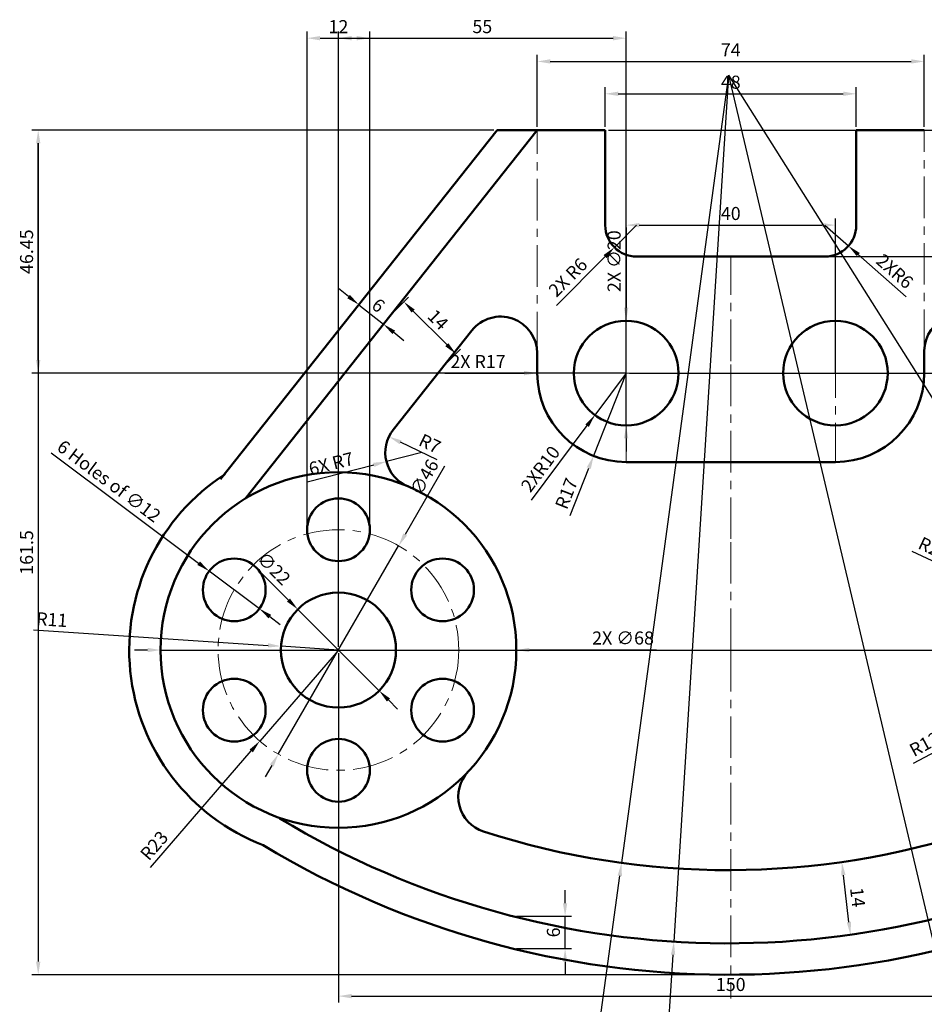
# Model space of a CAD drawing. Units: millimetres. Extents: x 2455 to 2735, y 1365 to 1648.
# Tile 2 of 3: x 2455 to 2628, y 1460 to 1648. Entities that reach past the tile are written whole.
import ezdxf

# ---------------------------------------------------------------- set-up
doc = ezdxf.new("R2010")
doc.units = ezdxf.units.MM
doc.linetypes.add('CENTER', pattern=[50.8, 31.75, -6.35, 6.35, -6.35])
for name, color, linetype, lineweight in [('M-CNTR', 4, 'CENTER', 18), ('M-DIMS', 2, 'Continuous', 25), ('M-OUTL', 7, 'Continuous', 50)]:
    doc.layers.add(name, color=color, linetype=linetype, lineweight=lineweight)
doc.styles.get("Standard").update_dxf_attribs({"font": 'arial.ttf'})
doc.dimstyles.new('ISO-25', dxfattribs={"dimtxt": 2.5, "dimasz": 2.5, "dimexe": 1.25, "dimexo": 0.625, "dimtad": 1, "dimdec": 0, "dimtxsty": 'Standard', "dimcen": 2.5, "dimadec": 0, "dimazin": 0, "dimtfac": 1, "dimtdec": 0, "dimtmove": 0, "dimatfit": 3, "dimfxl": 1, "dimarcsym": 0})

# ---------------------------------------------------------------- blocks, each defined once
blk = doc.blocks.new('*U1')
blk.add_circle((0, 0), 6)
blk = doc.blocks.new('*U2')
at = {"layer": 'M-OUTL', "color": 0, "linetype": 'ByBlock', "lineweight": -2, "transparency": 16777216}
blk.add_blockref('*U1', (2515.88, 1550.3), dxfattribs=at)
for p, rotation in [((2495.96, 1538.8), 59.99999999999999), ((2535.79, 1538.8), 300), ((2495.96, 1515.8), 120), ((2535.79, 1515.8), 240), ((2515.88, 1504.3), 180)]:
    blk.add_blockref('*U1', p, dxfattribs=dict(at, rotation=rotation))
blk = doc.blocks.new('*D3')
at = {"layer": 'Defpoints', "color": 0, "transparency": 16777216}
for p in [(2627.88, 1639.86), (2553.88, 1626.71), (2627.88, 1626.71)]:
    blk.add_point(p, dxfattribs=at)
at = {"layer": 'M-DIMS', "color": 0, "lineweight": -2, "transparency": 16777216}
for p, q in [((2553.88, 1627.33), (2553.88, 1641.11)), ((2627.88, 1627.33), (2627.88, 1641.11)), ((2556.38, 1639.86), (2625.38, 1639.86))]:
    blk.add_line(p, q, dxfattribs=at)
at = {"layer": 'M-DIMS', "color": 0, "transparency": 16777216}
for points in [[(2556.38, 1640.28), (2556.38, 1639.45), (2553.88, 1639.86)], [(2625.38, 1640.28), (2625.38, 1639.45), (2627.88, 1639.86)]]:
    blk.add_solid(points, dxfattribs=at)
at = {"layer": 'M-DIMS', "color": 0, "transparency": 16777216, "insert": (2590.88, 1641.74), "char_height": 2.5, "attachment_point": 5}
blk.add_mtext('74', dxfattribs=at)
blk = doc.blocks.new('*D4')
at = {"layer": 'Defpoints', "color": 0, "transparency": 16777216}
for p in [(2614.88, 1633.67), (2566.88, 1626.71), (2614.88, 1626.71)]:
    blk.add_point(p, dxfattribs=at)
at = {"layer": 'M-DIMS', "color": 0, "lineweight": -2, "transparency": 16777216}
for p, q in [((2566.88, 1627.33), (2566.88, 1634.92)), ((2614.88, 1627.33), (2614.88, 1634.92)), ((2569.38, 1633.67), (2612.38, 1633.67))]:
    blk.add_line(p, q, dxfattribs=at)
at = {"layer": 'M-DIMS', "color": 0, "transparency": 16777216}
for points in [[(2569.38, 1634.09), (2569.38, 1633.26), (2566.88, 1633.67)], [(2612.38, 1634.09), (2612.38, 1633.26), (2614.88, 1633.67)]]:
    blk.add_solid(points, dxfattribs=at)
at = {"layer": 'M-DIMS', "color": 0, "transparency": 16777216, "insert": (2590.88, 1635.57), "char_height": 2.5, "attachment_point": 5}
blk.add_mtext('48', dxfattribs=at)
blk = doc.blocks.new('*D5')
at = {"layer": 'Defpoints', "color": 0, "transparency": 16777216}
for p in [(2610.88, 1608.56), (2570.88, 1579.89), (2610.88, 1579.7)]:
    blk.add_point(p, dxfattribs=at)
at = {"layer": 'M-DIMS', "color": 0, "lineweight": -2, "transparency": 16777216}
for p, q in [((2570.88, 1580.52), (2570.88, 1609.81)), ((2573.38, 1608.56), (2608.38, 1608.56)), ((2610.88, 1580.33), (2610.88, 1609.81))]:
    blk.add_line(p, q, dxfattribs=at)
at = {"layer": 'M-DIMS', "color": 0, "transparency": 16777216}
for points in [[(2573.38, 1608.97), (2573.38, 1608.14), (2570.88, 1608.56)], [(2608.38, 1608.97), (2608.38, 1608.14), (2610.88, 1608.56)]]:
    blk.add_solid(points, dxfattribs=at)
at = {"layer": 'M-DIMS', "color": 0, "transparency": 16777216, "insert": (2590.88, 1610.46), "char_height": 2.5, "attachment_point": 5}
blk.add_mtext('40', dxfattribs=at)
blk = doc.blocks.new('*D6')
at = {"layer": 'Defpoints', "color": 0, "transparency": 16777216}
for p in [(2515.88, 1527.3), (2665.87, 1527.3), (2665.87, 1461.12)]:
    blk.add_point(p, dxfattribs=at)
at = {"layer": 'M-DIMS', "color": 0, "lineweight": -2, "transparency": 16777216}
for p, q in [((2515.88, 1526.68), (2515.88, 1459.87)), ((2665.87, 1526.68), (2665.87, 1459.87)), ((2518.38, 1461.12), (2663.37, 1461.12))]:
    blk.add_line(p, q, dxfattribs=at)
at = {"layer": 'M-DIMS', "color": 0, "transparency": 16777216}
for points in [[(2518.38, 1461.53), (2518.38, 1460.7), (2515.88, 1461.12)], [(2663.37, 1461.53), (2663.37, 1460.7), (2665.87, 1461.12)]]:
    blk.add_solid(points, dxfattribs=at)
at = {"layer": 'M-DIMS', "color": 0, "transparency": 16777216, "insert": (2590.87, 1463.02), "char_height": 2.5, "attachment_point": 5}
blk.add_mtext('150', dxfattribs=at)
blk = doc.blocks.new('*D7')
at = {"layer": 'Defpoints', "color": 0, "transparency": 16777216}
for p in [(2549.27, 1476.39), (2559.21, 1476.39), (2549.27, 1470.2)]:
    blk.add_point(p, dxfattribs=at)
at = {"layer": 'M-DIMS', "color": 0, "lineweight": -2, "transparency": 16777216}
for p, q in [((2559.21, 1478.89), (2559.21, 1481.39)), ((2549.9, 1476.39), (2560.46, 1476.39)), ((2559.21, 1470.2), (2559.21, 1476.39)), ((2549.9, 1470.2), (2560.46, 1470.2)), ((2559.21, 1467.7), (2559.21, 1465.2))]:
    blk.add_line(p, q, dxfattribs=at)
at = {"layer": 'M-DIMS', "color": 0, "transparency": 16777216}
for points in [[(2558.79, 1478.89), (2559.62, 1478.89), (2559.21, 1476.39)], [(2558.79, 1467.7), (2559.62, 1467.7), (2559.21, 1470.2)]]:
    blk.add_solid(points, dxfattribs=at)
at = {"layer": 'M-DIMS', "color": 0, "transparency": 16777216, "insert": (2557.3, 1473.3), "char_height": 2.5, "attachment_point": 5, "rotation": 90}
blk.add_mtext('6', dxfattribs=at)
blk = doc.blocks.new('*D8')
at = {"layer": 'Defpoints', "color": 0, "transparency": 16777216}
for p in [(2608.17, 1486.25), (2612.13, 1486.71), (2609.8, 1472.34)]:
    blk.add_point(p, dxfattribs=at)
at = {"layer": 'M-DIMS', "color": 0, "lineweight": -2, "transparency": 16777216}
for p, q in [((2608.79, 1486.32), (2613.37, 1486.86)), ((2613.47, 1475.29), (2612.42, 1484.23)), ((2610.43, 1472.42), (2615, 1472.95))]:
    blk.add_line(p, q, dxfattribs=at)
at = {"layer": 'M-DIMS', "color": 0, "transparency": 16777216}
for points in [[(2612.83, 1484.28), (2612, 1484.18), (2612.13, 1486.71)], [(2613.88, 1475.34), (2613.06, 1475.24), (2613.76, 1472.81)]]:
    blk.add_solid(points, dxfattribs=at)
at = {"layer": 'M-DIMS', "color": 0, "transparency": 16777216, "insert": (2614.81, 1479.98), "char_height": 2.5, "attachment_point": 5, "rotation": 276.7045}
blk.add_mtext('14', dxfattribs=at)
blk = doc.blocks.new('*D9')
at = {"layer": 'Defpoints', "color": 0, "transparency": 16777216}
for p in [(2525.95, 1591.48), (2538.34, 1583.94), (2535.92, 1581.51)]:
    blk.add_point(p, dxfattribs=at)
at = {"layer": 'M-DIMS', "color": 0, "lineweight": -2, "transparency": 16777216}
for p, q in [((2526.4, 1591.92), (2529.26, 1594.79)), ((2530.15, 1592.13), (2536.58, 1585.7)), ((2536.36, 1581.95), (2539.23, 1584.82))]:
    blk.add_line(p, q, dxfattribs=at)
at = {"layer": 'M-DIMS', "color": 0, "transparency": 16777216}
for points in [[(2530.44, 1592.43), (2529.85, 1591.84), (2528.38, 1593.9)], [(2536.87, 1586), (2536.28, 1585.41), (2538.34, 1583.94)]]:
    blk.add_solid(points, dxfattribs=at)
at = {"layer": 'M-DIMS', "color": 0, "transparency": 16777216, "insert": (2534.69, 1590.25), "char_height": 2.5, "attachment_point": 5, "rotation": 315}
blk.add_mtext('14', dxfattribs=at)
blk = doc.blocks.new('*D10')
at = {"layer": 'Defpoints', "color": 0, "transparency": 16777216}
for p in [(2519.78, 1593.34), (2524.48, 1589.61), (2524.48, 1589.61)]:
    blk.add_point(p, dxfattribs=at)
at = {"layer": 'M-DIMS', "color": 0, "lineweight": -2, "transparency": 16777216}
for p, q in [((2517.82, 1594.89), (2515.86, 1596.45)), ((2519.78, 1593.34), (2524.48, 1589.61)), ((2520.16, 1593.83), (2520.55, 1594.32)), ((2524.87, 1590.1), (2525.25, 1590.59)), ((2526.44, 1588.06), (2528.4, 1586.51))]:
    blk.add_line(p, q, dxfattribs=at)
at = {"layer": 'M-DIMS', "color": 0, "transparency": 16777216}
for points in [[(2518.07, 1595.22), (2517.56, 1594.57), (2519.78, 1593.34)], [(2526.7, 1588.39), (2526.18, 1587.73), (2524.48, 1589.61)]]:
    blk.add_solid(points, dxfattribs=at)
at = {"layer": 'M-DIMS', "color": 0, "transparency": 16777216, "insert": (2523.31, 1592.97), "char_height": 2.5, "attachment_point": 5, "rotation": 321.6022}
blk.add_mtext('6', dxfattribs=at)
blk = doc.blocks.new('*D11')
at = {"layer": 'Defpoints', "color": 0, "transparency": 16777216}
for p in [(2525.52, 1568.11), (2531.83, 1565.07)]:
    blk.add_point(p, dxfattribs=at)
at = {"layer": 'M-DIMS', "color": 0, "lineweight": -2, "transparency": 16777216}
blk.add_line((2534.78, 1563.65), (2527.77, 1567.03), dxfattribs=at)
at = {"layer": 'M-DIMS', "color": 0, "transparency": 16777216}
blk.add_solid([(2527.95, 1567.4), (2527.59, 1566.65), (2525.52, 1568.11)], dxfattribs=at)
at = {"layer": 'M-DIMS', "color": 0, "transparency": 16777216, "insert": (2533.22, 1566.49), "char_height": 2.5, "attachment_point": 5, "rotation": 334.2857}
blk.add_mtext('R7', dxfattribs=at)
blk = doc.blocks.new('*D12')
at = {"layer": 'Defpoints', "color": 0, "transparency": 16777216}
for p in [(2570.88, 1580.26), (2564.91, 1572.23)]:
    blk.add_point(p, dxfattribs=at)
at = {"layer": 'M-DIMS', "color": 0, "lineweight": -2, "transparency": 16777216}
for p, q in [((2570.88, 1580.26), (2564.91, 1572.23)), ((2552.8, 1555.94), (2563.42, 1570.23))]:
    blk.add_line(p, q, dxfattribs=at)
at = {"layer": 'M-DIMS', "color": 0, "transparency": 16777216}
blk.add_solid([(2563.08, 1570.47), (2563.75, 1569.98), (2564.91, 1572.23)], dxfattribs=at)
at = {"layer": 'M-DIMS', "color": 0, "transparency": 16777216, "insert": (2554.75, 1561.75), "char_height": 2.5, "attachment_point": 5, "rotation": 53.3711}
blk.add_mtext('2XR10', dxfattribs=at)
blk = doc.blocks.new('*D14')
at = {"layer": 'Defpoints', "color": 0, "transparency": 16777216}
for p in [(2570.88, 1580.26), (2564.66, 1564.44)]:
    blk.add_point(p, dxfattribs=at)
at = {"layer": 'M-DIMS', "color": 0, "lineweight": -2, "transparency": 16777216}
for p, q in [((2570.88, 1580.26), (2564.66, 1564.44)), ((2560.18, 1553.06), (2563.74, 1562.11))]:
    blk.add_line(p, q, dxfattribs=at)
at = {"layer": 'M-DIMS', "color": 0, "transparency": 16777216}
blk.add_solid([(2563.35, 1562.26), (2564.13, 1561.96), (2564.66, 1564.44)], dxfattribs=at)
at = {"layer": 'M-DIMS', "color": 0, "transparency": 16777216, "insert": (2559.76, 1557.11), "char_height": 2.5, "attachment_point": 5, "rotation": 68.5378}
blk.add_mtext('R17', dxfattribs=at)
blk = doc.blocks.new('*D15')
at = {"layer": 'Defpoints', "color": 0, "transparency": 16777216}
for p in [(2608.88, 1608.56), (2613.37, 1604.59)]:
    blk.add_point(p, dxfattribs=at)
at = {"layer": 'M-DIMS', "color": 0, "lineweight": -2, "transparency": 16777216}
for p, q in [((2608.88, 1608.56), (2613.37, 1604.59)), ((2624.42, 1594.84), (2615.25, 1602.93))]:
    blk.add_line(p, q, dxfattribs=at)
at = {"layer": 'M-DIMS', "color": 0, "transparency": 16777216}
blk.add_solid([(2615.53, 1603.24), (2614.97, 1602.62), (2613.37, 1604.59)], dxfattribs=at)
at = {"layer": 'M-DIMS', "color": 0, "transparency": 16777216, "insert": (2622.03, 1599.49), "char_height": 2.5, "attachment_point": 5, "rotation": 318.5765}
blk.add_mtext('2XR6', dxfattribs=at)
blk = doc.blocks.new('*D16')
at = {"layer": 'Defpoints', "color": 0, "transparency": 16777216}
for p in [(2647.76, 1535.78), (2665.88, 1527.3)]:
    blk.add_point(p, dxfattribs=at)
at = {"layer": 'M-DIMS', "color": 0, "lineweight": -2, "transparency": 16777216}
for p, q in [((2625.49, 1546.19), (2645.49, 1536.84)), ((2665.88, 1527.3), (2647.76, 1535.78))]:
    blk.add_line(p, q, dxfattribs=at)
at = {"layer": 'M-DIMS', "color": 0, "transparency": 16777216}
blk.add_solid([(2645.67, 1537.21), (2645.32, 1536.46), (2647.76, 1535.78)], dxfattribs=at)
at = {"layer": 'M-DIMS', "color": 0, "transparency": 16777216, "insert": (2629.56, 1546.39), "char_height": 2.5, "attachment_point": 5, "rotation": 334.9373}
blk.add_mtext('R20', dxfattribs=at)
blk = doc.blocks.new('*D17')
at = {"layer": 'Defpoints', "color": 0, "transparency": 16777216}
for p in [(2665.88, 1527.3), (2654.44, 1521.12)]:
    blk.add_point(p, dxfattribs=at)
at = {"layer": 'M-DIMS', "color": 0, "lineweight": -2, "transparency": 16777216}
for p, q in [((2665.88, 1527.3), (2654.44, 1521.12)), ((2625.82, 1505.64), (2652.24, 1519.93))]:
    blk.add_line(p, q, dxfattribs=at)
at = {"layer": 'M-DIMS', "color": 0, "transparency": 16777216}
blk.add_solid([(2652.04, 1520.3), (2652.44, 1519.56), (2654.44, 1521.12)], dxfattribs=at)
at = {"layer": 'M-DIMS', "color": 0, "transparency": 16777216, "insert": (2628.09, 1509.03), "char_height": 2.5, "attachment_point": 5, "rotation": 28.4115}
blk.add_mtext('R13', dxfattribs=at)
blk = doc.blocks.new('*D18')
at = {"layer": 'Defpoints', "color": 0, "transparency": 16777216}
for p in [(2515.88, 1527.3), (2500.84, 1509.9)]:
    blk.add_point(p, dxfattribs=at)
at = {"layer": 'M-DIMS', "color": 0, "lineweight": -2, "transparency": 16777216}
for p, q in [((2515.88, 1527.3), (2500.84, 1509.9)), ((2479.96, 1485.72), (2499.21, 1508.01))]:
    blk.add_line(p, q, dxfattribs=at)
at = {"layer": 'M-DIMS', "color": 0, "transparency": 16777216}
blk.add_solid([(2498.89, 1508.28), (2499.52, 1507.73), (2500.84, 1509.9)], dxfattribs=at)
at = {"layer": 'M-DIMS', "color": 0, "transparency": 16777216, "insert": (2480.89, 1489.7), "char_height": 2.5, "attachment_point": 5, "rotation": 49.1853}
blk.add_mtext('R23', dxfattribs=at)
blk = doc.blocks.new('*D19')
at = {"layer": 'Defpoints', "color": 0, "transparency": 16777216}
for p in [(2504.9, 1528.03), (2515.88, 1527.3)]:
    blk.add_point(p, dxfattribs=at)
at = {"layer": 'M-DIMS', "color": 0, "lineweight": -2, "transparency": 16777216}
for p, q in [((2457.59, 1531.14), (2502.41, 1528.19)), ((2515.88, 1527.3), (2504.9, 1528.03))]:
    blk.add_line(p, q, dxfattribs=at)
at = {"layer": 'M-DIMS', "color": 0, "transparency": 16777216}
blk.add_solid([(2502.43, 1528.61), (2502.38, 1527.78), (2504.9, 1528.03)], dxfattribs=at)
at = {"layer": 'M-DIMS', "color": 0, "transparency": 16777216, "insert": (2461.07, 1532.8), "char_height": 2.5, "attachment_point": 5, "rotation": 356.2348}
blk.add_mtext('R11', dxfattribs=at)
blk = doc.blocks.new('*D23')
at = {"layer": 'Defpoints', "color": 0, "transparency": 16777216}
for p in [(2590.42, 1637.21), (2682.22, 1491.75)]:
    blk.add_point(p, dxfattribs=at)
at = {"layer": 'M-DIMS', "color": 0, "lineweight": -2, "transparency": 16777216}
for p, q in [((2590.42, 1637.21), (2682.22, 1491.75)), ((2692.82, 1474.97), (2683.56, 1489.64))]:
    blk.add_line(p, q, dxfattribs=at)
blk.add_arc((2590.42, 1637.21), 172, 300.8351, 302.6735, dxfattribs=at)
at = {"layer": 'M-DIMS', "color": 0, "transparency": 16777216}
blk.add_solid([(2683.91, 1489.86), (2683.21, 1489.42), (2682.22, 1491.75)], dxfattribs=at)
at = {"layer": 'M-DIMS', "color": 0, "transparency": 16777216, "insert": (2691.97, 1479.84), "char_height": 2.5, "attachment_point": 5, "rotation": 302.2571}
blk.add_mtext('R172', dxfattribs=at)
blk = doc.blocks.new('*D24')
at = {"layer": 'Defpoints', "color": 0, "transparency": 16777216}
for p in [(2491.16, 1542.4), (2500.76, 1535.21)]:
    blk.add_point(p, dxfattribs=at)
at = {"layer": 'M-DIMS', "color": 0, "lineweight": -2, "transparency": 16777216}
for p, q in [((2460.94, 1565.04), (2489.15, 1543.9)), ((2500.76, 1535.21), (2491.16, 1542.4)), ((2502.76, 1533.71), (2504.76, 1532.21))]:
    blk.add_line(p, q, dxfattribs=at)
at = {"layer": 'M-DIMS', "color": 0, "transparency": 16777216}
for points in [[(2489.4, 1544.23), (2488.9, 1543.57), (2491.16, 1542.4)], [(2503.01, 1534.04), (2502.51, 1533.37), (2500.76, 1535.21)]]:
    blk.add_solid(points, dxfattribs=at)
at = {"layer": 'M-DIMS', "color": 0, "transparency": 16777216, "insert": (2471.82, 1559.35), "char_height": 2.5, "attachment_point": 5, "rotation": 323.1605}
blk.add_mtext('6 Holes of ∅12', dxfattribs=at)
blk = doc.blocks.new('MOUNT-HOLE-D20')
blk.add_circle((10, 10), 10)
blk = doc.blocks.new('*D26')
at = {"layer": 'Defpoints', "color": 0, "transparency": 16777216}
for p in [(2546.22, 1626.71), (2458.48, 1465.21), (2589.67, 1465.21)]:
    blk.add_point(p, dxfattribs=at)
at = {"layer": 'M-DIMS', "color": 0, "lineweight": -2, "transparency": 16777216}
for p, q in [((2545.6, 1626.71), (2457.23, 1626.71)), ((2458.48, 1624.21), (2458.48, 1467.71)), ((2589.05, 1465.21), (2457.23, 1465.21))]:
    blk.add_line(p, q, dxfattribs=at)
at = {"layer": 'M-DIMS', "color": 0, "transparency": 16777216}
for points in [[(2458.07, 1624.21), (2458.9, 1624.21), (2458.48, 1626.71)], [(2458.07, 1467.71), (2458.9, 1467.71), (2458.48, 1465.21)]]:
    blk.add_solid(points, dxfattribs=at)
at = {"layer": 'M-DIMS', "color": 0, "transparency": 16777216, "insert": (2456.58, 1545.96), "char_height": 2.5, "attachment_point": 5, "rotation": 90}
blk.add_mtext('161.5', dxfattribs=at)
blk = doc.blocks.new('*D27')
at = {"layer": 'Defpoints', "color": 0, "transparency": 16777216}
for p in [(2570.88, 1644.31), (2570.88, 1580.26), (2515.88, 1527.3)]:
    blk.add_point(p, dxfattribs=at)
at = {"layer": 'M-DIMS', "color": 0, "lineweight": -2, "transparency": 16777216}
for p, q in [((2515.88, 1527.93), (2515.88, 1645.56)), ((2518.38, 1644.31), (2568.38, 1644.31)), ((2570.88, 1580.88), (2570.88, 1645.56))]:
    blk.add_line(p, q, dxfattribs=at)
at = {"layer": 'M-DIMS', "color": 0, "transparency": 16777216}
for points in [[(2518.38, 1644.72), (2518.38, 1643.89), (2515.88, 1644.31)], [(2568.38, 1644.72), (2568.38, 1643.89), (2570.88, 1644.31)]]:
    blk.add_solid(points, dxfattribs=at)
at = {"layer": 'M-DIMS', "color": 0, "transparency": 16777216, "insert": (2543.38, 1646.2), "char_height": 2.5, "attachment_point": 5}
blk.add_mtext('55', dxfattribs=at)
blk = doc.blocks.new('*D28')
at = {"layer": 'Defpoints', "color": 0, "transparency": 16777216}
for p in [(2570.88, 1580.26), (2723.2, 1580.26), (2515.88, 1527.3)]:
    blk.add_point(p, dxfattribs=at)
at = {"layer": 'M-DIMS', "color": 0, "lineweight": -2, "transparency": 16777216}
for p, q in [((2571.5, 1580.26), (2724.45, 1580.26)), ((2723.2, 1529.8), (2723.2, 1577.76)), ((2516.5, 1527.3), (2724.45, 1527.3))]:
    blk.add_line(p, q, dxfattribs=at)
at = {"layer": 'M-DIMS', "color": 0, "transparency": 16777216}
for points in [[(2722.79, 1577.76), (2723.62, 1577.76), (2723.2, 1580.26)], [(2722.79, 1529.8), (2723.62, 1529.8), (2723.2, 1527.3)]]:
    blk.add_solid(points, dxfattribs=at)
at = {"layer": 'M-DIMS', "color": 0, "transparency": 16777216, "insert": (2721.3, 1553.78), "char_height": 2.5, "attachment_point": 5, "rotation": 90}
blk.add_mtext('52.95', dxfattribs=at)
blk = doc.blocks.new('*D29')
at = {"layer": 'Defpoints', "color": 0, "transparency": 16777216}
for p in [(2458.48, 1626.71), (2546.22, 1626.71), (2570.88, 1580.26)]:
    blk.add_point(p, dxfattribs=at)
at = {"layer": 'M-DIMS', "color": 0, "lineweight": -2, "transparency": 16777216}
for p, q in [((2545.6, 1626.71), (2457.23, 1626.71)), ((2458.48, 1582.76), (2458.48, 1624.21)), ((2570.25, 1580.26), (2457.23, 1580.26))]:
    blk.add_line(p, q, dxfattribs=at)
at = {"layer": 'M-DIMS', "color": 0, "transparency": 16777216}
for points in [[(2458.07, 1624.21), (2458.9, 1624.21), (2458.48, 1626.71)], [(2458.07, 1582.76), (2458.9, 1582.76), (2458.48, 1580.26)]]:
    blk.add_solid(points, dxfattribs=at)
at = {"layer": 'M-DIMS', "color": 0, "transparency": 16777216, "insert": (2456.58, 1603.48), "char_height": 2.5, "attachment_point": 5, "rotation": 90}
blk.add_mtext('46.45', dxfattribs=at)
blk = doc.blocks.new('*D30')
at = {"layer": 'Defpoints', "color": 0, "transparency": 16777216}
for p in [(2566.88, 1626.71), (2723.2, 1626.71), (2572.88, 1602.56)]:
    blk.add_point(p, dxfattribs=at)
at = {"layer": 'M-DIMS', "color": 0, "lineweight": -2, "transparency": 16777216}
for p, q in [((2567.5, 1626.71), (2724.45, 1626.71)), ((2723.2, 1605.06), (2723.2, 1624.21)), ((2573.5, 1602.56), (2724.45, 1602.56))]:
    blk.add_line(p, q, dxfattribs=at)
at = {"layer": 'M-DIMS', "color": 0, "transparency": 16777216}
for points in [[(2722.79, 1624.21), (2723.62, 1624.21), (2723.2, 1626.71)], [(2722.79, 1605.06), (2723.62, 1605.06), (2723.2, 1602.56)]]:
    blk.add_solid(points, dxfattribs=at)
at = {"layer": 'M-DIMS', "color": 0, "transparency": 16777216, "insert": (2721.3, 1614.63), "char_height": 2.5, "attachment_point": 5, "rotation": 90}
blk.add_mtext('24.153', dxfattribs=at)
blk = doc.blocks.new('*D31')
at = {"layer": 'Defpoints', "color": 0, "transparency": 16777216}
for p in [(2521.88, 1644.31), (2509.88, 1550.3), (2521.88, 1550.3)]:
    blk.add_point(p, dxfattribs=at)
at = {"layer": 'M-DIMS', "color": 0, "lineweight": -2, "transparency": 16777216}
for p, q in [((2509.88, 1550.93), (2509.88, 1645.56)), ((2512.38, 1644.31), (2519.38, 1644.31)), ((2521.88, 1550.93), (2521.88, 1645.56))]:
    blk.add_line(p, q, dxfattribs=at)
at = {"layer": 'M-DIMS', "color": 0, "transparency": 16777216}
for points in [[(2512.38, 1644.72), (2512.38, 1643.89), (2509.88, 1644.31)], [(2519.38, 1644.72), (2519.38, 1643.89), (2521.88, 1644.31)]]:
    blk.add_solid(points, dxfattribs=at)
at = {"layer": 'M-DIMS', "color": 0, "transparency": 16777216, "insert": (2515.88, 1646.19), "char_height": 2.5, "attachment_point": 5}
blk.add_mtext('12', dxfattribs=at)
blk = doc.blocks.new('*D32')
at = {"layer": 'Defpoints', "color": 0, "transparency": 16777216}
for p in [(2553.88, 1580.26), (2570.88, 1580.26)]:
    blk.add_point(p, dxfattribs=at)
at = {"layer": 'M-DIMS', "color": 0, "lineweight": -2, "transparency": 16777216}
for p, q in [((2536.24, 1580.26), (2551.38, 1580.26)), ((2570.88, 1580.26), (2553.88, 1580.26))]:
    blk.add_line(p, q, dxfattribs=at)
at = {"layer": 'M-DIMS', "color": 0, "transparency": 16777216}
blk.add_solid([(2551.38, 1580.67), (2551.38, 1579.84), (2553.88, 1580.26)], dxfattribs=at)
at = {"layer": 'M-DIMS', "color": 0, "transparency": 16777216, "insert": (2542.56, 1582.14), "char_height": 2.5, "attachment_point": 5, "rotation": 0.0002}
blk.add_mtext('2X R17', dxfattribs=at)
blk = doc.blocks.new('*D34')
at = {"layer": 'Defpoints', "color": 0, "transparency": 16777216}
for p in [(2481.88, 1527.3), (2549.88, 1527.3)]:
    blk.add_point(p, dxfattribs=at)
at = {"layer": 'M-DIMS', "color": 0, "lineweight": -2, "transparency": 16777216}
for p, q in [((2479.38, 1527.3), (2476.88, 1527.3)), ((2481.88, 1527.3), (2549.88, 1527.3)), ((2576.69, 1527.3), (2552.38, 1527.3))]:
    blk.add_line(p, q, dxfattribs=at)
at = {"layer": 'M-DIMS', "color": 0, "transparency": 16777216}
for points in [[(2479.38, 1527.72), (2479.38, 1526.89), (2481.88, 1527.3)], [(2552.38, 1527.72), (2552.38, 1526.89), (2549.88, 1527.3)]]:
    blk.add_solid(points, dxfattribs=at)
at = {"layer": 'M-DIMS', "color": 0, "transparency": 16777216, "insert": (2570.28, 1529.28), "char_height": 2.5, "attachment_point": 5, "rotation": 359.9994}
blk.add_mtext('2X ∅68', dxfattribs=at)
blk = doc.blocks.new('*D35')
at = {"layer": 'Defpoints', "color": 0, "transparency": 16777216}
for p in [(2527.38, 1547.22), (2504.38, 1507.39)]:
    blk.add_point(p, dxfattribs=at)
at = {"layer": 'M-DIMS', "color": 0, "lineweight": -2, "transparency": 16777216}
for p, q in [((2536.16, 1562.44), (2528.63, 1549.39)), ((2504.38, 1507.39), (2527.38, 1547.22)), ((2503.13, 1505.22), (2501.88, 1503.06))]:
    blk.add_line(p, q, dxfattribs=at)
at = {"layer": 'M-DIMS', "color": 0, "transparency": 16777216}
for points in [[(2528.27, 1549.6), (2528.99, 1549.18), (2527.38, 1547.22)], [(2502.76, 1505.43), (2503.49, 1505.01), (2504.38, 1507.39)]]:
    blk.add_solid(points, dxfattribs=at)
at = {"layer": 'M-DIMS', "color": 0, "transparency": 16777216, "insert": (2532.57, 1560.16), "char_height": 2.5, "attachment_point": 5, "rotation": 59.9998}
blk.add_mtext('∅46', dxfattribs=at)
blk = doc.blocks.new('*D36')
at = {"layer": 'Defpoints', "color": 0, "transparency": 16777216}
for p in [(2508.1, 1535.08), (2523.65, 1519.53)]:
    blk.add_point(p, dxfattribs=at)
at = {"layer": 'M-DIMS', "color": 0, "lineweight": -2, "transparency": 16777216}
for p, q in [((2499.24, 1543.94), (2506.33, 1536.85)), ((2523.65, 1519.53), (2508.1, 1535.08)), ((2525.42, 1517.76), (2527.19, 1515.99))]:
    blk.add_line(p, q, dxfattribs=at)
at = {"layer": 'M-DIMS', "color": 0, "transparency": 16777216}
for points in [[(2506.62, 1537.14), (2506.04, 1536.56), (2508.1, 1535.08)], [(2525.72, 1518.05), (2525.13, 1517.46), (2523.65, 1519.53)]]:
    blk.add_solid(points, dxfattribs=at)
at = {"layer": 'M-DIMS', "color": 0, "transparency": 16777216, "insert": (2503.3, 1542.67), "char_height": 2.5, "attachment_point": 5, "rotation": 315.0007}
blk.add_mtext('∅22', dxfattribs=at)
blk = doc.blocks.new('*D37')
at = {"layer": 'Defpoints', "color": 0, "transparency": 16777216}
for p in [(2570.88, 1590.26), (2570.88, 1570.26)]:
    blk.add_point(p, dxfattribs=at)
at = {"layer": 'M-DIMS', "color": 0, "lineweight": -2, "transparency": 16777216}
for p, q in [((2570.88, 1608.08), (2570.88, 1592.76)), ((2570.88, 1570.26), (2570.88, 1590.26)), ((2570.88, 1567.76), (2570.88, 1565.26))]:
    blk.add_line(p, q, dxfattribs=at)
at = {"layer": 'M-DIMS', "color": 0, "transparency": 16777216}
for points in [[(2570.46, 1592.76), (2571.29, 1592.76), (2570.88, 1590.26)], [(2570.46, 1567.76), (2571.29, 1567.76), (2570.88, 1570.26)]]:
    blk.add_solid(points, dxfattribs=at)
at = {"layer": 'M-DIMS', "color": 0, "transparency": 16777216, "insert": (2568.9, 1601.67), "char_height": 2.5, "attachment_point": 5, "rotation": 89.9992}
blk.add_mtext('2X ∅20', dxfattribs=at)
blk = doc.blocks.new('*D38')
at = {"layer": 'Defpoints', "color": 0, "transparency": 16777216}
for p in [(2531.83, 1565.07), (2525.04, 1563.34)]:
    blk.add_point(p, dxfattribs=at)
at = {"layer": 'M-DIMS', "color": 0, "lineweight": -2, "transparency": 16777216}
for p, q in [((2531.83, 1565.07), (2525.04, 1563.34)), ((2509.87, 1559.45), (2522.62, 1562.72))]:
    blk.add_line(p, q, dxfattribs=at)
at = {"layer": 'M-DIMS', "color": 0, "transparency": 16777216}
blk.add_solid([(2522.52, 1563.12), (2522.73, 1562.32), (2525.04, 1563.34)], dxfattribs=at)
at = {"layer": 'M-DIMS', "color": 0, "transparency": 16777216, "insert": (2514.56, 1562.62), "char_height": 2.5, "attachment_point": 5, "rotation": 14.358}
blk.add_mtext('6X R7', dxfattribs=at)
blk = doc.blocks.new('*D39')
at = {"layer": 'Defpoints', "color": 0, "transparency": 16777216}
for p in [(2572.88, 1608.56), (2568.63, 1604.31)]:
    blk.add_point(p, dxfattribs=at)
at = {"layer": 'M-DIMS', "color": 0, "lineweight": -2, "transparency": 16777216}
for p, q in [((2572.88, 1608.56), (2568.63, 1604.31)), ((2557.54, 1593.21), (2566.87, 1602.54))]:
    blk.add_line(p, q, dxfattribs=at)
at = {"layer": 'M-DIMS', "color": 0, "transparency": 16777216}
blk.add_solid([(2566.57, 1602.84), (2567.16, 1602.25), (2568.63, 1604.31)], dxfattribs=at)
at = {"layer": 'M-DIMS', "color": 0, "transparency": 16777216, "insert": (2559.97, 1598.34), "char_height": 2.5, "attachment_point": 5, "rotation": 45.0012}
blk.add_mtext('2X R6', dxfattribs=at)
blk = doc.blocks.new('*D40')
at = {"layer": 'Defpoints', "color": 0, "transparency": 16777216}
for p in [(2590.42, 1637.21), (2629.97, 1469.82)]:
    blk.add_point(p, dxfattribs=at)
at = {"layer": 'M-DIMS', "color": 0, "lineweight": -2, "transparency": 16777216}
for p, q in [((2590.42, 1637.21), (2629.97, 1469.82)), ((2654.75, 1364.93), (2630.55, 1467.38))]:
    blk.add_line(p, q, dxfattribs=at)
at = {"layer": 'M-DIMS', "color": 0, "transparency": 16777216}
blk.add_solid([(2630.95, 1467.48), (2630.14, 1467.29), (2629.97, 1469.82)], dxfattribs=at)
at = {"layer": 'M-DIMS', "color": 0, "transparency": 16777216, "insert": (2655.53, 1369.81), "char_height": 2.5, "attachment_point": 5, "rotation": 283.2931}
blk.add_mtext('R172', dxfattribs=at)
blk = doc.blocks.new('*D41')
at = {"layer": 'Defpoints', "color": 0, "transparency": 16777216}
for p in [(2590.42, 1637.21), (2569.99, 1486.59)]:
    blk.add_point(p, dxfattribs=at)
at = {"layer": 'M-DIMS', "color": 0, "lineweight": -2, "transparency": 16777216}
for p, q in [((2590.42, 1637.21), (2569.99, 1486.59)), ((2557.12, 1391.69), (2569.66, 1484.11))]:
    blk.add_line(p, q, dxfattribs=at)
at = {"layer": 'M-DIMS', "color": 0, "transparency": 16777216}
blk.add_solid([(2569.24, 1484.17), (2570.07, 1484.05), (2569.99, 1486.59)], dxfattribs=at)
at = {"layer": 'M-DIMS', "color": 0, "transparency": 16777216, "insert": (2555.85, 1396.47), "char_height": 2.5, "attachment_point": 5, "rotation": 82.2752}
blk.add_mtext('R152', dxfattribs=at)
blk = doc.blocks.new('*D42')
at = {"layer": 'Defpoints', "color": 0, "transparency": 16777216}
for p in [(2590.42, 1637.21), (2580, 1471.54)]:
    blk.add_point(p, dxfattribs=at)
at = {"layer": 'M-DIMS', "color": 0, "lineweight": -2, "transparency": 16777216}
for p, q in [((2590.42, 1637.21), (2580, 1471.54)), ((2573.46, 1367.56), (2579.84, 1469.04))]:
    blk.add_line(p, q, dxfattribs=at)
at = {"layer": 'M-DIMS', "color": 0, "transparency": 16777216}
blk.add_solid([(2579.43, 1469.07), (2580.26, 1469.01), (2580, 1471.54)], dxfattribs=at)
at = {"layer": 'M-DIMS', "color": 0, "transparency": 16777216, "insert": (2571.85, 1372.25), "char_height": 2.5, "attachment_point": 5, "rotation": 86.3994}
blk.add_mtext('R166', dxfattribs=at)

msp = doc.modelspace()

# ---------------------------------------------------------------- linework, layer by layer
at = {"layer": 'M-CNTR', "ltscale": 0.25, "transparency": 33554534}
for p, q in [((2553.8759, 1584.0653), (2553.8759, 1626.7079)), ((2627.8759, 1584.4896), (2627.8759, 1626.7079)), ((2590.8759, 1582.555), (2590.8759, 1602.555)), ((2570.8759, 1596.53), (2570.8759, 1563.2571)), ((2610.8759, 1596.1431), (2610.8759, 1563.2571)), ((2590.8759, 1548.555), (2590.8759, 1582.555)), ((2553.8759, 1580.2571), (2627.8759, 1580.2571)), ((2590.8759, 1527.3043), (2590.8759, 1548.555)), ((2481.8759, 1527.3043), (2699.8759, 1527.3043)), ((2590.8759, 1527.3043), (2590.8759, 1460.6833))]:
    msp.add_line(p, q, dxfattribs=at)
msp.add_circle((2515.8759, 1527.3043), 23, dxfattribs=at)
at = {"layer": 'M-OUTL'}
for p, q in [((2493.3308, 1559.973), (2546.22, 1626.7079)), ((2498.0331, 1556.2463), (2553.8759, 1626.7079)), ((2553.8759, 1626.7079), (2546.22, 1626.7079)), ((2566.8759, 1626.7079), (2553.8759, 1626.7079)), ((2566.8759, 1608.555), (2566.8759, 1626.7079)), ((2614.8759, 1608.555), (2614.8759, 1626.7079)), ((2614.8759, 1626.7079), (2627.8759, 1626.7079)), ((2590.8759, 1602.555), (2572.8759, 1602.555)), ((2590.8759, 1602.555), (2608.8759, 1602.555)), ((2526.3394, 1569.4227), (2541.3898, 1588.4132)), ((2553.8759, 1584.0653), (2553.8759, 1580.2571)), ((2627.8759, 1580.2571), (2627.8759, 1584.4896)), ((2627.8759, 1584.4896), (2627.8759, 1580.2571)), ((2570.8759, 1563.2571), (2610.8759, 1563.2571))]:
    msp.add_line(p, q, dxfattribs=at)
for radius in [34, 11]:
    msp.add_circle((2515.8759, 1527.3043), radius, dxfattribs=at)
for centre, radius, start, end in [((2572.8759, 1608.555), 6, 180, 270), ((2608.8759, 1608.555), 6, 270, 0), ((2634.8759, 1584.4896), 7, 38.801949, 180), ((2546.8759, 1584.0653), 7, 0, 141.602201), ((2570.8759, 1580.2571), 17, 180, 270), ((2610.8759, 1580.2571), 17, 270, 0), ((2531.8254, 1565.0749), 7, 141.602201, 247.106928), ((2515.8759, 1527.3043), 40, 122.742885, 248.948482), ((2545.7775, 1499.2527), 7, 136.828355, 252.066838), ((2590.424, 1637.2081), 166, 238.871706, 300.62686), ((2590.424, 1637.2081), 152, 252.066838, 288.221236), ((2590.424, 1637.2081), 172, 238.871706, 300.62686)]:
    msp.add_arc(centre, radius, start, end, dxfattribs=at)

# ---------------------------------------------------------------- block references
for name, p in [('MOUNT-HOLE-D20', (2560.876, 1570.257)), ('MOUNT-HOLE-D20', (2600.876, 1570.257)), ('*U2', (0, 0))]:
    msp.add_blockref(name, p, dxfattribs=at)

# ---------------------------------------------------------------- dimensions: what is measured, and where the dimension line sits
at = {"layer": 'M-DIMS'}
for base, p1, p2, override, picture, middle in [((2521.8759, 1644.3079), (2509.8759, 1550.3043), (2521.8759, 1550.3043), {"dimdec": 0, "dimlfac": 1, "dimrnd": 0, "dimzin": 0, "dimdsep": 46, "dimlunit": 2}, '*D31', (2515.8759, 1646.188)), ((2570.8759, 1644.3079), (2515.8759, 1527.3043), (2570.8759, 1580.2571), {"dimdec": 0, "dimlfac": 1, "dimrnd": 0, "dimzin": 0, "dimdsep": 46, "dimlunit": 2}, '*D27', (2543.3759, 1646.2042)), ((2627.8759, 1639.8623), (2553.8759, 1626.7079), (2627.8759, 1626.7079), {"dimclrd": 0, "dimclre": 0, "dimclrt": 0}, '*D3', (2590.8759, 1641.7373)), ((2614.8759, 1633.672), (2566.8759, 1626.7079), (2614.8759, 1626.7079), {"dimclrd": 0, "dimclre": 0, "dimclrt": 0}, '*D4', (2590.8759, 1635.5734)), ((2610.8759, 1608.555), (2570.8759, 1579.8935), (2610.8759, 1579.7001), {"dimclrd": 0, "dimclre": 0, "dimclrt": 0}, '*D5', (2590.8759, 1610.4565)), ((2665.8712, 1461.1167), (2515.8759, 1527.3043), (2665.8712, 1527.3043), {"dimclrd": 0, "dimclre": 0, "dimclrt": 0}, '*D6', (2590.8735, 1463.0182))]:
    dim = msp.add_linear_dim(base=base, p1=p1, p2=p2, dimstyle='ISO-25', override=override, dxfattribs=at)
    dim.commit()
    dim.dimension.update_dxf_attribs({"geometry": picture, "text_midpoint": middle})
for center, mpoint, override, picture, middle in [((2590.424, 1637.2081), (2569.9929, 1486.5875), {"dimdec": 0, "dimlfac": 1, "dimrnd": 0, "dimzin": 0, "dimdsep": 46, "dimlunit": 2}, '*D41', (2557.7342, 1396.2151)), ((2590.424, 1637.2081), (2579.9991, 1471.5357), {"dimdec": 0, "dimlfac": 1, "dimrnd": 0, "dimzin": 0, "dimdsep": 46, "dimlunit": 2}, '*D42', (2573.7441, 1372.1323)), ((2590.424, 1637.2081), (2682.2237, 1491.7543), {"dimclrd": 0, "dimclre": 0, "dimclrt": 0}, '*D23', (2690.3772, 1478.8354)), ((2590.424, 1637.2081), (2629.9725, 1469.8165), {"dimdec": 0, "dimlfac": 1, "dimrnd": 0, "dimzin": 0, "dimdsep": 46, "dimlunit": 2}, '*D40', (2653.7015, 1369.3816)), ((2531.8254, 1565.0749), (2525.5186, 1568.1121), {"dimclrd": 0, "dimclre": 0, "dimclrt": 0}, '*D11', (2532.4026, 1564.7969)), ((2665.8759, 1527.3043), (2647.759, 1535.7765), {"dimclrd": 0, "dimclre": 0, "dimclrt": 0}, '*D16', (2628.753, 1544.6645)), ((2515.8759, 1527.3043), (2504.8996, 1528.0267), {"dimclrd": 0, "dimclre": 0, "dimclrt": 0}, '*D19', (2460.9504, 1530.919)), ((2515.8759, 1527.3043), (2500.8427, 1509.8973), {"dimclrd": 0, "dimclre": 0, "dimclrt": 0}, '*D18', (2482.325, 1488.4553)), ((2665.8759, 1527.3043), (2654.4417, 1521.1189), {"dimclrd": 0, "dimclre": 0, "dimclrt": 0}, '*D17', (2628.9987, 1507.3554))]:
    dim = msp.add_radius_dim(center=center, mpoint=mpoint, dimstyle='ISO-25', override=override, dxfattribs=at)
    dim.commit()
    dim.dimension.update_dxf_attribs({"geometry": picture, "text_midpoint": middle, "dimtype": 164})
for base, p1, p2, override, picture, middle in [((2458.4839, 1465.2097), (2546.22, 1626.7079), (2589.6714, 1465.2097), {"dimdec": 1, "dimlfac": 1, "dimrnd": 0, "dimzin": 0, "dimdsep": 46, "dimlunit": 2}, '*D26', (2456.5824, 1545.9588)), ((2458.4839, 1626.7079), (2570.8759, 1580.2571), (2546.22, 1626.7079), {"dimdec": 2, "dimlfac": 1, "dimrnd": 0, "dimzin": 0, "dimdsep": 46, "dimlunit": 2}, '*D29', (2456.5824, 1603.4825)), ((2723.204, 1626.7079), (2572.8759, 1602.555), (2566.8759, 1626.7079), {"dimdec": 3, "dimlfac": 1, "dimrnd": 0, "dimzin": 0, "dimdsep": 46, "dimlunit": 2}, '*D30', (2721.3017, 1614.6315)), ((2723.204, 1580.2571), (2515.8759, 1527.3043), (2570.8759, 1580.2571), {"dimdec": 2, "dimlfac": 1, "dimrnd": 0, "dimzin": 0, "dimdsep": 46, "dimlunit": 2}, '*D28', (2721.3025, 1553.7807))]:
    dim = msp.add_linear_dim(base=base, p1=p1, p2=p2, angle=90, dimstyle='ISO-25', override=override, dxfattribs=at)
    dim.commit()
    dim.dimension.update_dxf_attribs({"geometry": picture, "text_midpoint": middle})
for center, mpoint, text, override, picture, middle in [((2572.8759, 1608.555), (2568.6333, 1604.3123), '2X <>', {"dimdec": 0, "dimlfac": 1, "dimrnd": 0, "dimzin": 0, "dimdsep": 46, "dimlunit": 2}, '*D39', (2559.9725, 1598.3402)), ((2608.8759, 1608.555), (2613.3749, 1604.5853), '2X<>', {"dimclrd": 0, "dimclre": 0, "dimclrt": 0}, '*D15', (2622.0278, 1599.4863)), ((2570.8759, 1580.2571), (2553.8759, 1580.257), '2X <>', {"dimdec": 0, "dimlfac": 1, "dimrnd": 0, "dimzin": 0, "dimdsep": 46, "dimlunit": 2}, '*D32', (2542.5568, 1582.1379)), ((2531.8254, 1565.0749), (2525.044, 1563.339), '6X <>', {"dimdec": 0, "dimlfac": 1, "dimrnd": 0, "dimzin": 0, "dimdsep": 46, "dimlunit": 2}, '*D38', (2514.5619, 1562.6186))]:
    dim = msp.add_radius_dim(center=center, mpoint=mpoint, text=text, dimstyle='ISO-25', override=override, dxfattribs=at)
    dim.commit()
    dim.dimension.update_dxf_attribs({"geometry": picture, "text_midpoint": middle})
dim = msp.add_diameter_dim_2p(p1=(2570.8757, 1570.2571), p2=(2570.876, 1590.2571), text='2X <>', dimstyle='ISO-25', override={"dimdec": 0, "dimlfac": 1, "dimrnd": 0, "dimzin": 0, "dimdsep": 46, "dimlunit": 2}, dxfattribs=at)
dim.commit()
dim.dimension.update_dxf_attribs({"geometry": '*D37', "text_midpoint": (2570.8762, 1601.6691)})
for p1, p2, distance, picture, middle in [((2519.7754, 1593.3404), (2524.4777, 1589.6137), 0, '*D10', (2523.3076, 1592.9673)), ((2525.9545, 1591.4771), (2535.9201, 1581.5115), 3.4282, '*D9', (2534.6908, 1590.2478)), ((2609.8044, 1472.3433), (2608.1699, 1486.2475), -3.9842, '*D8', (2614.8113, 1479.9801)), ((2549.2735, 1470.2032), (2549.2735, 1476.3894), -9.9323, '*D7', (2557.3044, 1473.2963))]:
    dim = msp.add_aligned_dim(p1=p1, p2=p2, distance=distance, dimstyle='ISO-25', override={"dimclrd": 0, "dimclre": 0, "dimclrt": 0}, dxfattribs=at)
    dim.commit()
    dim.dimension.update_dxf_attribs({"geometry": picture, "text_midpoint": middle})
dim = msp.add_radius_dim(center=(2570.8759, 1580.2571), mpoint=(2564.9096, 1572.2319), text='2X<>', dimstyle='ISO-25', override={"dimclrd": 0, "dimclre": 0, "dimclrt": 0}, dxfattribs=at)
dim.commit()
dim.dimension.update_dxf_attribs({"geometry": '*D12', "text_midpoint": (2556.276, 1560.619), "dimtype": 164})
dim = msp.add_radius_dim(center=(2570.8759, 1580.2571), mpoint=(2564.6558, 1564.4359), dimstyle='ISO-25', override={"dimclrd": 0, "dimclre": 0, "dimclrt": 0}, dxfattribs=at)
dim.commit()
dim.dimension.update_dxf_attribs({"geometry": '*D14', "text_midpoint": (2559.7551, 1557.109)})
for p1, p2, text, override, picture, middle in [((2500.7592, 1535.2069), (2491.1554, 1542.4018), '6 Holes of <>', {"dimclrd": 0, "dimclre": 0, "dimclrt": 0}, '*D24', (2470.6368, 1557.7737)), ((2481.8759, 1527.3047), (2549.8759, 1527.304), '2X <>', {"dimdec": 0, "dimlfac": 1, "dimrnd": 0, "dimzin": 0, "dimdsep": 46, "dimlunit": 2}, '*D34', (2570.2759, 1527.3038))]:
    dim = msp.add_diameter_dim_2p(p1=p1, p2=p2, text=text, dimstyle='ISO-25', override=override, dxfattribs=at)
    dim.commit()
    dim.dimension.update_dxf_attribs({"geometry": picture, "text_midpoint": middle, "dimtype": 163})
dim = msp.add_diameter_dim_2p(p1=(2504.3758, 1507.3858), p2=(2527.3759, 1547.2229), dimstyle='ISO-25', override={"dimdec": 0, "dimlfac": 1, "dimrnd": 0, "dimzin": 0, "dimdsep": 46, "dimlunit": 2}, dxfattribs=at)
dim.commit()
dim.dimension.update_dxf_attribs({"geometry": '*D35', "text_midpoint": (2534.276, 1559.174), "dimtype": 163})
dim = msp.add_diameter_dim_2p(p1=(2523.6541, 1519.5263), p2=(2508.0976, 1535.0824), dimstyle='ISO-25', override={"dimdec": 0, "dimlfac": 1, "dimrnd": 0, "dimzin": 0, "dimdsep": 46, "dimlunit": 2}, dxfattribs=at)
dim.commit()
dim.dimension.update_dxf_attribs({"geometry": '*D36', "text_midpoint": (2501.9013, 1541.2786)})

doc.saveas('drawing.dxf')
